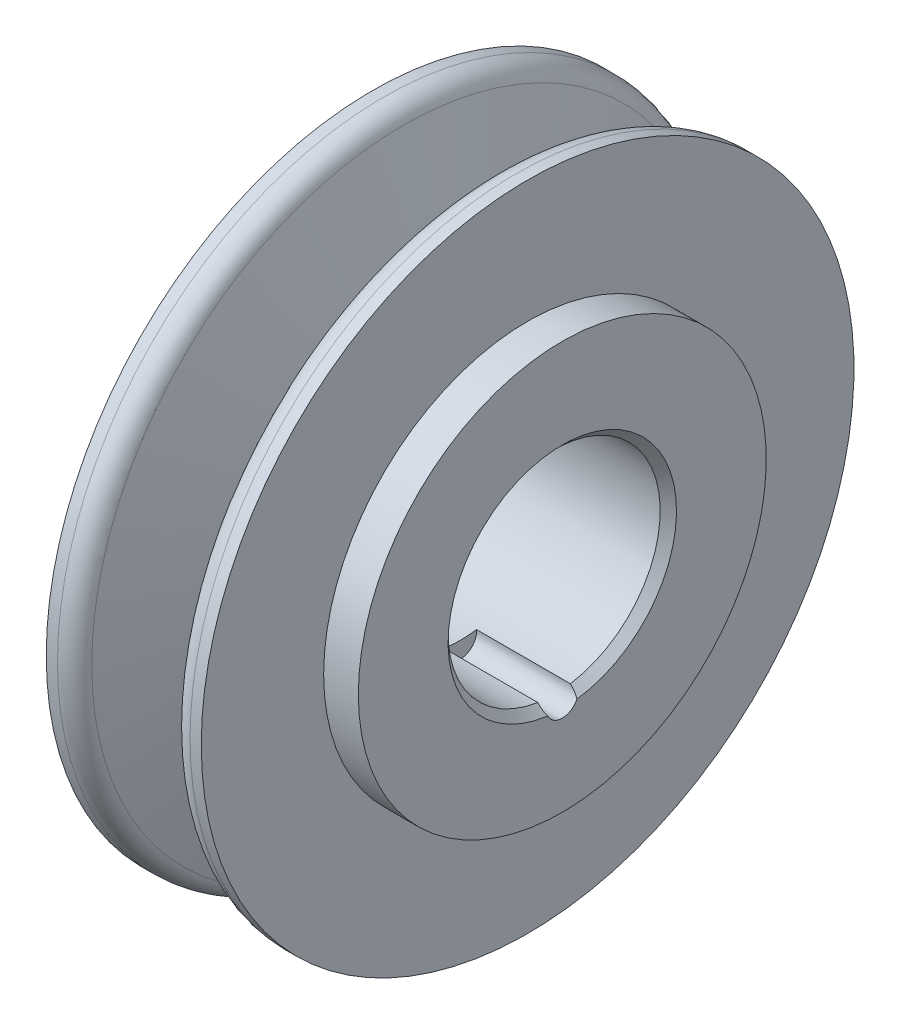
ISO-10303-21;
HEADER;
FILE_DESCRIPTION(('STEP AP214'),'2;1');
FILE_NAME('part.step','',(''),(''),'','','');
FILE_SCHEMA(('AUTOMOTIVE_DESIGN { 1 0 10303 214 1 1 1 1 }'));
ENDSEC;
DATA;
#1=APPLICATION_CONTEXT('core data for automotive mechanical design processes');
#2=APPLICATION_PROTOCOL_DEFINITION('international standard','automotive_design',2000,#1);
#3=PRODUCT_CONTEXT('',#1,'mechanical');
#4=PRODUCT('Part','Part','',(#3));
#5=PRODUCT_RELATED_PRODUCT_CATEGORY('part','',(#4));
#6=PRODUCT_DEFINITION_FORMATION('','',#4);
#7=PRODUCT_DEFINITION_CONTEXT('part definition',#1,'design');
#8=PRODUCT_DEFINITION('design','',#6,#7);
#9=PRODUCT_DEFINITION_SHAPE('','',#8);
#10=(LENGTH_UNIT() NAMED_UNIT(*) SI_UNIT(.MILLI.,.METRE.));
#11=(NAMED_UNIT(*) PLANE_ANGLE_UNIT() SI_UNIT($,.RADIAN.));
#12=(NAMED_UNIT(*) SI_UNIT($,.STERADIAN.) SOLID_ANGLE_UNIT());
#13=UNCERTAINTY_MEASURE_WITH_UNIT(LENGTH_MEASURE(1.E-05),#10,'distance_accuracy_value','');
#14=(GEOMETRIC_REPRESENTATION_CONTEXT(3) GLOBAL_UNCERTAINTY_ASSIGNED_CONTEXT((#13)) GLOBAL_UNIT_ASSIGNED_CONTEXT((#10,
#11,#12)) REPRESENTATION_CONTEXT('',''));
#15=CARTESIAN_POINT('',(0.,0.,0.));
#16=DIRECTION('',(0.,0.,1.));
#17=DIRECTION('',(1.,0.,0.));
#18=AXIS2_PLACEMENT_3D('',#15,#16,#17);
#19=CARTESIAN_POINT('',(27.5,26.,0.));
#20=DIRECTION('',(-1.,0.,0.));
#21=DIRECTION('',(0.,0.,1.));
#22=AXIS2_PLACEMENT_3D('',#19,#20,#21);
#23=PLANE('',#22);
#24=CARTESIAN_POINT('',(27.5,0.,0.));
#25=DIRECTION('',(-1.,0.,0.));
#26=DIRECTION('',(0.,0.,1.));
#27=AXIS2_PLACEMENT_3D('',#24,#25,#26);
#28=CIRCLE('',#27,28.);
#29=CARTESIAN_POINT('',(27.5,-27.7692307692307,3.58745348195725));
#30=VERTEX_POINT('',#29);
#31=CARTESIAN_POINT('',(27.5,-27.7692307692307,-3.58745348195725));
#32=VERTEX_POINT('',#31);
#33=EDGE_CURVE('E81',#30,#32,#28,.T.);
#34=ORIENTED_EDGE('',*,*,#33,.T.);
#35=CARTESIAN_POINT('',(27.5,-26.,0.));
#36=DIRECTION('',(1.,0.,0.));
#37=DIRECTION('',(0.,0.,-1.));
#38=AXIS2_PLACEMENT_3D('',#35,#36,#37);
#39=CIRCLE('',#38,4.);
#40=EDGE_CURVE('E73',#30,#32,#39,.T.);
#41=ORIENTED_EDGE('',*,*,#40,.F.);
#42=EDGE_LOOP('',(#34,#41));
#43=FACE_BOUND('',#42,.T.);
#44=CARTESIAN_POINT('',(27.5,0.,0.));
#45=DIRECTION('',(-1.,0.,0.));
#46=DIRECTION('',(0.,0.,1.));
#47=AXIS2_PLACEMENT_3D('',#44,#45,#46);
#48=CIRCLE('',#47,50.);
#49=CARTESIAN_POINT('',(27.5,0.,50.));
#50=VERTEX_POINT('',#49);
#51=EDGE_CURVE('E89',#50,#50,#48,.T.);
#52=ORIENTED_EDGE('',*,*,#51,.F.);
#53=EDGE_LOOP('',(#52));
#54=FACE_BOUND('',#53,.T.);
#55=ADVANCED_FACE('F41',(#43,#54),#23,.F.);
#56=CARTESIAN_POINT('',(0.,0.,0.));
#57=DIRECTION('',(-1.,0.,0.));
#58=DIRECTION('',(0.,0.,1.));
#59=AXIS2_PLACEMENT_3D('',#56,#57,#58);
#60=CYLINDRICAL_SURFACE('',#59,50.);
#61=CARTESIAN_POINT('',(19.,0.,0.));
#62=DIRECTION('',(-1.,0.,0.));
#63=DIRECTION('',(0.,0.,1.));
#64=AXIS2_PLACEMENT_3D('',#61,#62,#63);
#65=CIRCLE('',#64,50.);
#66=CARTESIAN_POINT('',(19.,0.,50.));
#67=VERTEX_POINT('',#66);
#68=EDGE_CURVE('E96',#67,#67,#65,.T.);
#69=ORIENTED_EDGE('',*,*,#68,.F.);
#70=EDGE_LOOP('',(#69));
#71=FACE_BOUND('',#70,.T.);
#72=ORIENTED_EDGE('',*,*,#51,.T.);
#73=EDGE_LOOP('',(#72));
#74=FACE_BOUND('',#73,.T.);
#75=ADVANCED_FACE('F170',(#71,#74),#60,.T.);
#76=CARTESIAN_POINT('',(19.,50.,0.));
#77=DIRECTION('',(-1.,0.,0.));
#78=DIRECTION('',(0.,0.,1.));
#79=AXIS2_PLACEMENT_3D('',#76,#77,#78);
#80=PLANE('',#79);
#81=CARTESIAN_POINT('',(19.,0.,0.));
#82=DIRECTION('',(-1.,0.,0.));
#83=DIRECTION('',(0.,0.,1.));
#84=AXIS2_PLACEMENT_3D('',#81,#82,#83);
#85=CIRCLE('',#84,80.);
#86=CARTESIAN_POINT('',(19.,0.,80.));
#87=VERTEX_POINT('',#86);
#88=EDGE_CURVE('E325',#87,#87,#85,.T.);
#89=ORIENTED_EDGE('',*,*,#88,.F.);
#90=EDGE_LOOP('',(#89));
#91=FACE_BOUND('',#90,.T.);
#92=ORIENTED_EDGE('',*,*,#68,.T.);
#93=EDGE_LOOP('',(#92));
#94=FACE_BOUND('',#93,.T.);
#95=ADVANCED_FACE('F162',(#91,#94),#80,.F.);
#96=CARTESIAN_POINT('',(0.,0.,0.));
#97=DIRECTION('',(-1.,0.,0.));
#98=DIRECTION('',(0.,0.,1.));
#99=AXIS2_PLACEMENT_3D('',#96,#97,#98);
#100=CYLINDRICAL_SURFACE('',#99,80.);
#101=CARTESIAN_POINT('',(16.25,0.,0.));
#102=DIRECTION('',(-1.,0.,0.));
#103=DIRECTION('',(0.,0.,1.));
#104=AXIS2_PLACEMENT_3D('',#101,#102,#103);
#105=CIRCLE('',#104,80.);
#106=CARTESIAN_POINT('',(16.25,0.,80.));
#107=VERTEX_POINT('',#106);
#108=EDGE_CURVE('E317',#107,#107,#105,.T.);
#109=ORIENTED_EDGE('',*,*,#108,.F.);
#110=EDGE_LOOP('',(#109));
#111=FACE_BOUND('',#110,.T.);
#112=ORIENTED_EDGE('',*,*,#88,.T.);
#113=EDGE_LOOP('',(#112));
#114=FACE_BOUND('',#113,.T.);
#115=ADVANCED_FACE('F157',(#111,#114),#100,.T.);
#116=CARTESIAN_POINT('',(16.25,0.,0.));
#117=DIRECTION('',(-1.,0.,0.));
#118=DIRECTION('',(0.,0.,1.));
#119=AXIS2_PLACEMENT_3D('',#116,#117,#118);
#120=TOROIDAL_SURFACE('',#119,75.,4.99999999999999);
#121=CARTESIAN_POINT('',(11.45,0.,0.));
#122=DIRECTION('',(-1.,0.,0.));
#123=DIRECTION('',(0.,0.,1.));
#124=AXIS2_PLACEMENT_3D('',#121,#122,#123);
#125=CIRCLE('',#124,76.4);
#126=CARTESIAN_POINT('',(11.45,0.,76.4));
#127=VERTEX_POINT('',#126);
#128=EDGE_CURVE('E316',#127,#127,#125,.T.);
#129=ORIENTED_EDGE('',*,*,#128,.F.);
#130=EDGE_LOOP('',(#129));
#131=FACE_BOUND('',#130,.T.);
#132=ORIENTED_EDGE('',*,*,#108,.T.);
#133=EDGE_LOOP('',(#132));
#134=FACE_BOUND('',#133,.T.);
#135=ADVANCED_FACE('F154',(#131,#134),#120,.T.);
#136=CARTESIAN_POINT('',(11.45,0.,0.));
#137=DIRECTION('',(1.,0.,0.));
#138=DIRECTION('',(0.,0.,-1.));
#139=AXIS2_PLACEMENT_3D('',#136,#137,#138);
#140=CONICAL_SURFACE('',#139,76.4,1.28700221758657);
#141=CARTESIAN_POINT('',(4.8,0.,0.));
#142=DIRECTION('',(-1.,0.,0.));
#143=DIRECTION('',(0.,0.,1.));
#144=AXIS2_PLACEMENT_3D('',#141,#142,#143);
#145=CIRCLE('',#144,53.6);
#146=CARTESIAN_POINT('',(4.8,0.,53.6));
#147=VERTEX_POINT('',#146);
#148=EDGE_CURVE('E311',#147,#147,#145,.T.);
#149=ORIENTED_EDGE('',*,*,#148,.F.);
#150=EDGE_LOOP('',(#149));
#151=FACE_BOUND('',#150,.T.);
#152=ORIENTED_EDGE('',*,*,#128,.T.);
#153=EDGE_LOOP('',(#152));
#154=FACE_BOUND('',#153,.T.);
#155=ADVANCED_FACE('F151',(#151,#154),#140,.T.);
#156=CARTESIAN_POINT('',(0.,0.,0.));
#157=DIRECTION('',(-1.,0.,0.));
#158=DIRECTION('',(0.,0.,1.));
#159=AXIS2_PLACEMENT_3D('',#156,#157,#158);
#160=TOROIDAL_SURFACE('',#159,55.,5.);
#161=CARTESIAN_POINT('',(-4.8,0.,0.));
#162=DIRECTION('',(-1.,0.,0.));
#163=DIRECTION('',(0.,0.,1.));
#164=AXIS2_PLACEMENT_3D('',#161,#162,#163);
#165=CIRCLE('',#164,53.6);
#166=CARTESIAN_POINT('',(-4.8,0.,53.6));
#167=VERTEX_POINT('',#166);
#168=EDGE_CURVE('E309',#167,#167,#165,.T.);
#169=ORIENTED_EDGE('',*,*,#168,.F.);
#170=EDGE_LOOP('',(#169));
#171=FACE_BOUND('',#170,.T.);
#172=ORIENTED_EDGE('',*,*,#148,.T.);
#173=EDGE_LOOP('',(#172));
#174=FACE_BOUND('',#173,.T.);
#175=ADVANCED_FACE('F150',(#171,#174),#160,.F.);
#176=CARTESIAN_POINT('',(-4.8,0.,0.));
#177=DIRECTION('',(-1.,0.,0.));
#178=DIRECTION('',(0.,0.,1.));
#179=AXIS2_PLACEMENT_3D('',#176,#177,#178);
#180=CONICAL_SURFACE('',#179,53.6,1.28700221758657);
#181=CARTESIAN_POINT('',(-11.45,0.,0.));
#182=DIRECTION('',(-1.,0.,0.));
#183=DIRECTION('',(0.,0.,1.));
#184=AXIS2_PLACEMENT_3D('',#181,#182,#183);
#185=CIRCLE('',#184,76.4);
#186=CARTESIAN_POINT('',(-11.45,0.,76.4));
#187=VERTEX_POINT('',#186);
#188=EDGE_CURVE('E307',#187,#187,#185,.T.);
#189=ORIENTED_EDGE('',*,*,#188,.F.);
#190=EDGE_LOOP('',(#189));
#191=FACE_BOUND('',#190,.T.);
#192=ORIENTED_EDGE('',*,*,#168,.T.);
#193=EDGE_LOOP('',(#192));
#194=FACE_BOUND('',#193,.T.);
#195=ADVANCED_FACE('F141',(#191,#194),#180,.T.);
#196=CARTESIAN_POINT('',(-16.25,0.,0.));
#197=DIRECTION('',(-1.,0.,0.));
#198=DIRECTION('',(0.,0.,1.));
#199=AXIS2_PLACEMENT_3D('',#196,#197,#198);
#200=TOROIDAL_SURFACE('',#199,75.,4.99999999999999);
#201=CARTESIAN_POINT('',(-16.25,0.,0.));
#202=DIRECTION('',(-1.,0.,0.));
#203=DIRECTION('',(0.,0.,1.));
#204=AXIS2_PLACEMENT_3D('',#201,#202,#203);
#205=CIRCLE('',#204,80.);
#206=CARTESIAN_POINT('',(-16.25,0.,80.));
#207=VERTEX_POINT('',#206);
#208=EDGE_CURVE('E305',#207,#207,#205,.T.);
#209=ORIENTED_EDGE('',*,*,#208,.F.);
#210=EDGE_LOOP('',(#209));
#211=FACE_BOUND('',#210,.T.);
#212=ORIENTED_EDGE('',*,*,#188,.T.);
#213=EDGE_LOOP('',(#212));
#214=FACE_BOUND('',#213,.T.);
#215=ADVANCED_FACE('F140',(#211,#214),#200,.T.);
#216=CARTESIAN_POINT('',(0.,0.,0.));
#217=DIRECTION('',(-1.,0.,0.));
#218=DIRECTION('',(0.,0.,1.));
#219=AXIS2_PLACEMENT_3D('',#216,#217,#218);
#220=CYLINDRICAL_SURFACE('',#219,80.);
#221=CARTESIAN_POINT('',(-19.,0.,0.));
#222=DIRECTION('',(-1.,0.,0.));
#223=DIRECTION('',(0.,0.,1.));
#224=AXIS2_PLACEMENT_3D('',#221,#222,#223);
#225=CIRCLE('',#224,80.);
#226=CARTESIAN_POINT('',(-19.,0.,80.));
#227=VERTEX_POINT('',#226);
#228=EDGE_CURVE('E296',#227,#227,#225,.T.);
#229=ORIENTED_EDGE('',*,*,#228,.F.);
#230=EDGE_LOOP('',(#229));
#231=FACE_BOUND('',#230,.T.);
#232=ORIENTED_EDGE('',*,*,#208,.T.);
#233=EDGE_LOOP('',(#232));
#234=FACE_BOUND('',#233,.T.);
#235=ADVANCED_FACE('F132',(#231,#234),#220,.T.);
#236=CARTESIAN_POINT('',(-19.,50.,0.));
#237=DIRECTION('',(1.,0.,0.));
#238=DIRECTION('',(0.,0.,-1.));
#239=AXIS2_PLACEMENT_3D('',#236,#237,#238);
#240=PLANE('',#239);
#241=CARTESIAN_POINT('',(-19.,0.,0.));
#242=DIRECTION('',(-1.,0.,0.));
#243=DIRECTION('',(0.,0.,1.));
#244=AXIS2_PLACEMENT_3D('',#241,#242,#243);
#245=CIRCLE('',#244,50.);
#246=CARTESIAN_POINT('',(-19.,0.,50.));
#247=VERTEX_POINT('',#246);
#248=EDGE_CURVE('E291',#247,#247,#245,.T.);
#249=ORIENTED_EDGE('',*,*,#248,.F.);
#250=EDGE_LOOP('',(#249));
#251=FACE_BOUND('',#250,.T.);
#252=ORIENTED_EDGE('',*,*,#228,.T.);
#253=EDGE_LOOP('',(#252));
#254=FACE_BOUND('',#253,.T.);
#255=ADVANCED_FACE('F134',(#251,#254),#240,.F.);
#256=CARTESIAN_POINT('',(0.,0.,0.));
#257=DIRECTION('',(-1.,0.,0.));
#258=DIRECTION('',(0.,0.,1.));
#259=AXIS2_PLACEMENT_3D('',#256,#257,#258);
#260=CYLINDRICAL_SURFACE('',#259,50.);
#261=CARTESIAN_POINT('',(-27.5,0.,0.));
#262=DIRECTION('',(-1.,0.,0.));
#263=DIRECTION('',(0.,0.,1.));
#264=AXIS2_PLACEMENT_3D('',#261,#262,#263);
#265=CIRCLE('',#264,50.);
#266=CARTESIAN_POINT('',(-27.5,0.,50.));
#267=VERTEX_POINT('',#266);
#268=EDGE_CURVE('E295',#267,#267,#265,.T.);
#269=ORIENTED_EDGE('',*,*,#268,.F.);
#270=EDGE_LOOP('',(#269));
#271=FACE_BOUND('',#270,.T.);
#272=ORIENTED_EDGE('',*,*,#248,.T.);
#273=EDGE_LOOP('',(#272));
#274=FACE_BOUND('',#273,.T.);
#275=ADVANCED_FACE('F130',(#271,#274),#260,.T.);
#276=CARTESIAN_POINT('',(-27.5,26.,0.));
#277=DIRECTION('',(1.,0.,0.));
#278=DIRECTION('',(0.,0.,-1.));
#279=AXIS2_PLACEMENT_3D('',#276,#277,#278);
#280=PLANE('',#279);
#281=CARTESIAN_POINT('',(-27.5,0.,0.));
#282=DIRECTION('',(1.,0.,0.));
#283=DIRECTION('',(0.,0.,-1.));
#284=AXIS2_PLACEMENT_3D('',#281,#282,#283);
#285=CIRCLE('',#284,28.);
#286=CARTESIAN_POINT('',(-27.5,0.,-28.));
#287=VERTEX_POINT('',#286);
#288=EDGE_CURVE('E77',#287,#287,#285,.T.);
#289=ORIENTED_EDGE('',*,*,#288,.T.);
#290=EDGE_LOOP('',(#289));
#291=FACE_BOUND('',#290,.T.);
#292=ORIENTED_EDGE('',*,*,#268,.T.);
#293=EDGE_LOOP('',(#292));
#294=FACE_BOUND('',#293,.T.);
#295=ADVANCED_FACE('F122',(#291,#294),#280,.F.);
#296=CARTESIAN_POINT('',(0.,0.,0.));
#297=DIRECTION('',(-1.,0.,0.));
#298=DIRECTION('',(0.,0.,1.));
#299=AXIS2_PLACEMENT_3D('',#296,#297,#298);
#300=CYLINDRICAL_SURFACE('',#299,26.);
#301=CARTESIAN_POINT('',(25.5,0.,0.));
#302=DIRECTION('',(-1.,0.,0.));
#303=DIRECTION('',(0.,0.,1.));
#304=AXIS2_PLACEMENT_3D('',#301,#302,#303);
#305=CIRCLE('',#304,26.);
#306=CARTESIAN_POINT('',(25.5,-25.6923076923077,-3.98814812209715));
#307=VERTEX_POINT('',#306);
#308=CARTESIAN_POINT('',(25.5,-25.6923076923077,3.98814812209715));
#309=VERTEX_POINT('',#308);
#310=EDGE_CURVE('E91',#307,#309,#305,.F.);
#311=ORIENTED_EDGE('',*,*,#310,.T.);
#312=DIRECTION('',(1.,0.,0.));
#313=VECTOR('',#312,1.);
#314=CARTESIAN_POINT('',(15.,-25.6923076923077,3.98814812209714));
#315=LINE('',#314,#313);
#316=CARTESIAN_POINT('',(2.5,-25.6923076923077,3.98814812209714));
#317=VERTEX_POINT('',#316);
#318=EDGE_CURVE('E60',#309,#317,#315,.F.);
#319=ORIENTED_EDGE('',*,*,#318,.T.);
#320=CARTESIAN_POINT('',(2.5,0.,0.));
#321=DIRECTION('',(1.,0.,0.));
#322=DIRECTION('',(0.,0.,-1.));
#323=AXIS2_PLACEMENT_3D('',#320,#321,#322);
#324=CIRCLE('',#323,26.);
#325=CARTESIAN_POINT('',(2.5,-25.6923076923077,-3.98814812209714));
#326=VERTEX_POINT('',#325);
#327=EDGE_CURVE('E11',#326,#317,#324,.F.);
#328=ORIENTED_EDGE('',*,*,#327,.F.);
#329=DIRECTION('',(1.,0.,0.));
#330=VECTOR('',#329,1.);
#331=CARTESIAN_POINT('',(15.,-25.6923076923077,-3.98814812209714));
#332=LINE('',#331,#330);
#333=EDGE_CURVE('E294',#326,#307,#332,.T.);
#334=ORIENTED_EDGE('',*,*,#333,.T.);
#335=EDGE_LOOP('',(#311,#319,#328,#334));
#336=FACE_BOUND('',#335,.T.);
#337=CARTESIAN_POINT('',(-25.5,0.,0.));
#338=DIRECTION('',(1.,0.,0.));
#339=DIRECTION('',(0.,0.,-1.));
#340=AXIS2_PLACEMENT_3D('',#337,#338,#339);
#341=CIRCLE('',#340,26.);
#342=CARTESIAN_POINT('',(-25.5,0.,-26.));
#343=VERTEX_POINT('',#342);
#344=EDGE_CURVE('E90',#343,#343,#341,.F.);
#345=ORIENTED_EDGE('',*,*,#344,.T.);
#346=EDGE_LOOP('',(#345));
#347=FACE_BOUND('',#346,.T.);
#348=ADVANCED_FACE('F118',(#336,#347),#300,.F.);
#349=CARTESIAN_POINT('',(27.5,0.,0.));
#350=DIRECTION('',(1.,0.,0.));
#351=DIRECTION('',(0.,0.,-1.));
#352=AXIS2_PLACEMENT_3D('',#349,#350,#351);
#353=CONICAL_SURFACE('',#352,28.,0.785398163397451);
#354=CARTESIAN_POINT('',(27.5002,-27.7694461546154,-3.58734725192822));
#355=CARTESIAN_POINT('',(27.3912034838156,-27.6520584601297,-3.64522604699244));
#356=CARTESIAN_POINT('',(27.2803176472308,-27.5333331528356,-3.69664810402793));
#357=CARTESIAN_POINT('',(27.0555104334495,-27.2941078985508,-3.78703929419991));
#358=CARTESIAN_POINT('',(26.9415902182154,-27.1736086385516,-3.82601312195843));
#359=CARTESIAN_POINT('',(26.7128883473842,-26.9332377619489,-3.89157725219692));
#360=CARTESIAN_POINT('',(26.5981377424269,-26.8133787442407,-3.91832372726584));
#361=CARTESIAN_POINT('',(26.3668927670475,-26.5733954662483,-3.96056307795136));
#362=CARTESIAN_POINT('',(26.2503986121998,-26.4532712402949,-3.97605733326297));
#363=CARTESIAN_POINT('',(26.02878581011,-26.2262608013377,-3.99504065265693));
#364=CARTESIAN_POINT('',(25.9237930878251,-26.1193420420806,-3.99964283822895));
#365=CARTESIAN_POINT('',(25.7125238268727,-25.9054835108222,-4.00031865329183));
#366=CARTESIAN_POINT('',(25.6062433655611,-25.7985474367956,-3.99634111625742));
#367=CARTESIAN_POINT('',(25.4998,-25.6921076930769,-3.98813268677681));
#368=B_SPLINE_CURVE_WITH_KNOTS('',3,(#354,#355,#356,#357,#358,#359,#360,#361,#362,#363,#364,
#365,#366,#367),.UNSPECIFIED.,.F.,.F.,(4,2,2,2,2,2,4),(0.,0.510741271313679,1.02128969783997,
1.52512132528178,2.0288911647898,2.47841169048431,2.93062041092365),.UNSPECIFIED.);
#369=EDGE_CURVE('E49',#32,#307,#368,.T.);
#370=ORIENTED_EDGE('',*,*,#369,.F.);
#371=ORIENTED_EDGE('',*,*,#33,.F.);
#372=CARTESIAN_POINT('',(25.4998,-25.6921076930769,3.98813268677681));
#373=CARTESIAN_POINT('',(25.6515097306643,-25.8438034350887,3.99981081245395));
#374=CARTESIAN_POINT('',(25.802915253744,-25.996547998704,4.0029265330355));
#375=CARTESIAN_POINT('',(26.1043804543524,-26.3032783456437,3.99145302744375));
#376=CARTESIAN_POINT('',(26.2544369047565,-26.457265977499,3.97682901794202));
#377=CARTESIAN_POINT('',(26.5491139423541,-26.7621770814808,3.92968522861125));
#378=CARTESIAN_POINT('',(26.6937837382048,-26.9131045848054,3.89750119964121));
#379=CARTESIAN_POINT('',(26.9792877601105,-27.2132872129011,3.814726622015));
#380=CARTESIAN_POINT('',(27.1201265229038,-27.3625441805038,3.76415896328593));
#381=CARTESIAN_POINT('',(27.2991110201806,-27.553632845013,3.68624837749902));
#382=CARTESIAN_POINT('',(27.3395985117903,-27.5969542712243,3.66769369615966));
#383=CARTESIAN_POINT('',(27.4202092395352,-27.6833934275026,3.62883417619638));
#384=CARTESIAN_POINT('',(27.4603311821991,-27.7265102806359,3.60852470552495));
#385=CARTESIAN_POINT('',(27.5002,-27.7694461546154,3.58734725192825));
#386=B_SPLINE_CURVE_WITH_KNOTS('',3,(#372,#373,#374,#375,#376,#377,#378,#379,#380,#381,#382,
#383,#384,#385),.UNSPECIFIED.,.F.,.F.,(4,2,2,2,2,2,4),(0.,0.644495099612309,1.29025594375644,
1.92408162934315,2.55712081027836,2.74349507597593,2.93037728490115),.UNSPECIFIED.);
#387=EDGE_CURVE('E75',#309,#30,#386,.T.);
#388=ORIENTED_EDGE('',*,*,#387,.F.);
#389=ORIENTED_EDGE('',*,*,#310,.F.);
#390=EDGE_LOOP('',(#370,#371,#388,#389));
#391=FACE_BOUND('',#390,.T.);
#392=ADVANCED_FACE('F86',(#391),#353,.F.);
#393=CARTESIAN_POINT('',(-25.5,0.,0.));
#394=DIRECTION('',(-1.,0.,0.));
#395=DIRECTION('',(0.,0.,1.));
#396=AXIS2_PLACEMENT_3D('',#393,#394,#395);
#397=CONICAL_SURFACE('',#396,26.,0.785398163397453);
#398=ORIENTED_EDGE('',*,*,#288,.F.);
#399=EDGE_LOOP('',(#398));
#400=FACE_BOUND('',#399,.T.);
#401=ORIENTED_EDGE('',*,*,#344,.F.);
#402=EDGE_LOOP('',(#401));
#403=FACE_BOUND('',#402,.T.);
#404=ADVANCED_FACE('F42',(#400,#403),#397,.F.);
#405=CARTESIAN_POINT('',(2.5,-26.,0.));
#406=DIRECTION('',(1.,0.,0.));
#407=DIRECTION('',(0.,0.,-1.));
#408=AXIS2_PLACEMENT_3D('',#405,#406,#407);
#409=PLANE('',#408);
#410=ORIENTED_EDGE('',*,*,#327,.T.);
#411=CARTESIAN_POINT('',(2.5,-26.,0.));
#412=DIRECTION('',(1.,0.,0.));
#413=DIRECTION('',(0.,0.,-1.));
#414=AXIS2_PLACEMENT_3D('',#411,#412,#413);
#415=CIRCLE('',#414,4.);
#416=EDGE_CURVE('E88',#317,#326,#415,.T.);
#417=ORIENTED_EDGE('',*,*,#416,.T.);
#418=EDGE_LOOP('',(#410,#417));
#419=FACE_BOUND('',#418,.T.);
#420=ADVANCED_FACE('F120',(#419),#409,.T.);
#421=CARTESIAN_POINT('',(2.5,-26.,0.));
#422=DIRECTION('',(1.,0.,0.));
#423=DIRECTION('',(0.,0.,-1.));
#424=AXIS2_PLACEMENT_3D('',#421,#422,#423);
#425=CYLINDRICAL_SURFACE('',#424,4.);
#426=ORIENTED_EDGE('',*,*,#416,.F.);
#427=ORIENTED_EDGE('',*,*,#318,.F.);
#428=ORIENTED_EDGE('',*,*,#387,.T.);
#429=ORIENTED_EDGE('',*,*,#40,.T.);
#430=ORIENTED_EDGE('',*,*,#369,.T.);
#431=ORIENTED_EDGE('',*,*,#333,.F.);
#432=EDGE_LOOP('',(#426,#427,#428,#429,#430,#431));
#433=FACE_BOUND('',#432,.T.);
#434=ADVANCED_FACE('F74',(#433),#425,.F.);
#435=CLOSED_SHELL('',(#55,#75,#95,#115,#135,#155,#175,#195,#215,#235,#255,#275,#295,#348,#392,
#404,#420,#434));
#436=MANIFOLD_SOLID_BREP('B2',#435);
#437=ADVANCED_BREP_SHAPE_REPRESENTATION('',(#18,#436),#14);
#438=SHAPE_DEFINITION_REPRESENTATION(#9,#437);
ENDSEC;
END-ISO-10303-21;
